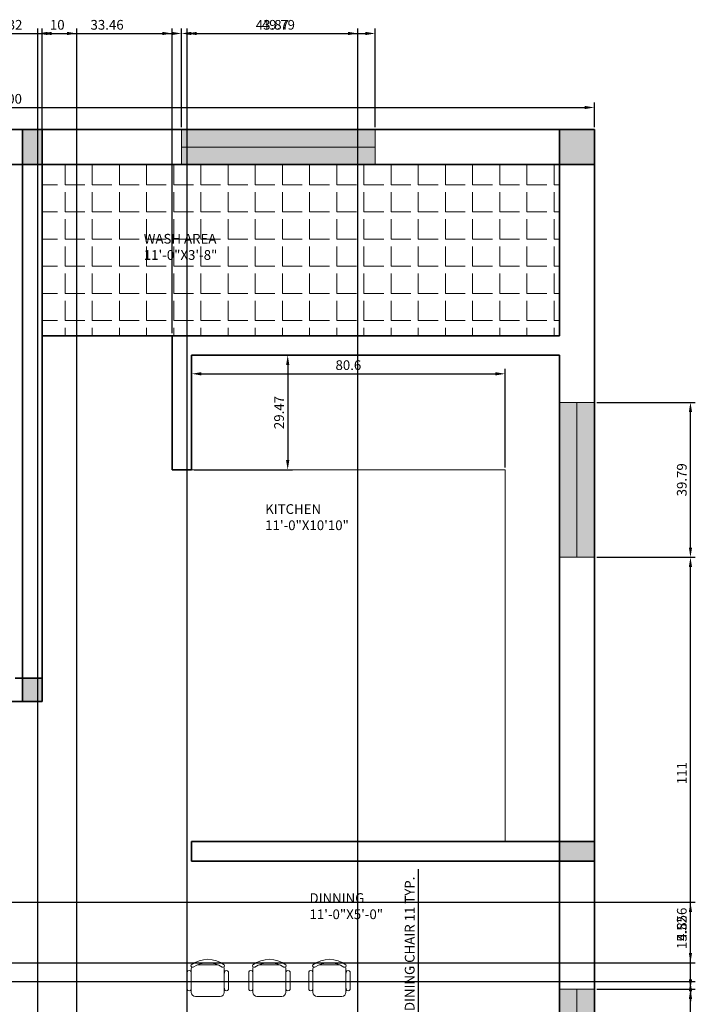
# Model space of a CAD drawing. Units: inches. Extents: x 33934 to 34340, y 20959 to 21493.
# Tile 4 of 4: x 34166 to 34340, y 21240 to 21493. Entities that reach past the tile are written whole.
import ezdxf

# ---------------------------------------------------------------- set-up
doc = ezdxf.new("R2010")
doc.units = ezdxf.units.IN
for name, color, linetype, lineweight in [('A-ANNO-DIMS', 2, 'Continuous', 18), ('A-AREA-IDEN', 7, 'Continuous', 18), ('A-FLOR-CASE', 9, 'Continuous', 18), ('A-FURN', 8, 'Continuous', 18), ('A-GLAZ', 4, 'Continuous', 18), ('A-WALL', 7, 'Continuous', 35)]:
    doc.layers.add(name, color=color, linetype=linetype, lineweight=lineweight)
for name, color, linetype, lineweight, true_color in [('A-COLS-PATT', 141, 'Continuous', 13, 0xadddf7), ('A-FLOR-PATT', 141, 'Continuous', 13, 0xadddf7), ('A-GLAZ-PATT', 159, 'Continuous', 13, 0x22346e)]:
    doc.layers.add(name, color=color, linetype=linetype, lineweight=lineweight, true_color=true_color)
doc.styles.get("Standard").update_dxf_attribs({"font": 'arial.ttf'})
doc.dimstyles.new('ISO-25', dxfattribs={"dimtxt": 2.5, "dimasz": 2.5, "dimexe": 1.25, "dimexo": 0.625, "dimtad": 1, "dimtxsty": 'Standard', "dimcen": 2.5, "dimadec": 0, "dimazin": 0, "dimtfac": 1, "dimtmove": 0, "dimatfit": 3, "dimfxl": 1, "dimarcsym": 0})

# ---------------------------------------------------------------- blocks, each defined once
blk = doc.blocks.new('CHAIR7')
for p, q in [((5.12, 15.04), (17.88, 15.04)), ((0, 9), (0, -9)), ((20, 12), (3, 12)), ((23, -7.44), (23, 7.44)), ((3, -12), (20, -12)), ((5.12, -15), (17.88, -15))]:
    blk.add_line(p, q)
for centre, radius, start, end in [((5.56, 13.54), 1.56, 73.7398, 286.2602), ((17.44, 13.54), 1.56, 253.7398, 106.2602), ((3, 9), 3, 90, 180), ((20, 9), 3, 62.41556, 90), ((22.34, 11.12), 1.1, 53.30994, 212.02741), ((4.82, 0), 19.64, 327.57575, 32.42425), ((7, 0), 20, 323.1301, 36.8699), ((3, -9), 3, 180, 270), ((5.56, -13.5), 1.56, 73.7398, 286.2602), ((17.44, -13.5), 1.56, 253.7398, 106.2602), ((20, -9), 3, 270, 297.58444), ((22.34, -11.12), 1.1, 147.97259, 306.69006)]:
    blk.add_arc(centre, radius, start, end)
blk = doc.blocks.new('*D6')
at = {"layer": 'A-ANNO-DIMS', "color": 0, "lineweight": -2, "transparency": 16777216}
for p, q in [((34013.69, 21465.74), (34013.69, 21472.03)), ((34313.69, 21465.74), (34313.69, 21472.03)), ((34016.19, 21470.78), (34311.19, 21470.78))]:
    blk.add_line(p, q, dxfattribs=at)
at = {"layer": 'A-ANNO-DIMS', "color": 0, "transparency": 16777216}
for points in [[(34016.19, 21471.2), (34016.19, 21470.37), (34013.69, 21470.78)], [(34311.19, 21471.2), (34311.19, 21470.37), (34313.69, 21470.78)]]:
    blk.add_solid(points, dxfattribs=at)
at = {"layer": 'Defpoints', "color": 0, "transparency": 16777216}
for p in [(34313.69, 21470.78), (34013.69, 21465.11), (34313.69, 21465.11)]:
    blk.add_point(p, dxfattribs=at)
at = {"layer": 'A-ANNO-DIMS', "color": 0, "transparency": 16777216, "insert": (34163.69, 21472.69), "char_height": 2.5, "attachment_point": 5}
blk.add_mtext('300', dxfattribs=at)
blk = doc.blocks.new('*D11')
at = {"layer": 'A-ANNO-DIMS', "color": 0, "lineweight": -2, "transparency": 16777216}
for p, q in [((34268.45, 21234.15), (34268.45, 21274.98)), ((34267.46, 21234.15), (34269.7, 21234.15)), ((34268.45, 21225.89), (34268.45, 21231.65)), ((34267.46, 21223.39), (34269.7, 21223.39))]:
    blk.add_line(p, q, dxfattribs=at)
at = {"layer": 'A-ANNO-DIMS', "color": 0, "transparency": 16777216}
for points in [[(34268.03, 21231.65), (34268.87, 21231.65), (34268.45, 21234.15)], [(34268.03, 21225.89), (34268.87, 21225.89), (34268.45, 21223.39)]]:
    blk.add_solid(points, dxfattribs=at)
at = {"layer": 'Defpoints', "color": 0, "transparency": 16777216}
for p in [(34266.83, 21234.15), (34268.45, 21234.15), (34266.83, 21223.39)]:
    blk.add_point(p, dxfattribs=at)
at = {"layer": 'A-ANNO-DIMS', "color": 0, "transparency": 16777216, "insert": (34266.53, 21255.82), "char_height": 2.5, "attachment_point": 5, "rotation": 90}
blk.add_mtext('DINING CHAIR 11 TYP.', dxfattribs=at)
blk = doc.blocks.new('*D15')
at = {"layer": 'A-ANNO-DIMS', "color": 0, "lineweight": -2, "transparency": 16777216}
for p, q in [((34117.23, 21465.74), (34117.23, 21491.06)), ((34119.73, 21489.81), (34205.05, 21489.81)), ((34207.55, 21465.74), (34207.55, 21491.06))]:
    blk.add_line(p, q, dxfattribs=at)
at = {"layer": 'A-ANNO-DIMS', "color": 0, "transparency": 16777216}
for points in [[(34119.73, 21490.23), (34119.73, 21489.39), (34117.23, 21489.81)], [(34205.05, 21490.23), (34205.05, 21489.39), (34207.55, 21489.81)]]:
    blk.add_solid(points, dxfattribs=at)
at = {"layer": 'Defpoints', "color": 0, "transparency": 16777216}
for p in [(34207.55, 21489.81), (34117.23, 21465.11), (34207.55, 21465.11)]:
    blk.add_point(p, dxfattribs=at)
at = {"layer": 'A-ANNO-DIMS', "color": 0, "transparency": 16777216, "insert": (34162.39, 21491.71), "char_height": 2.5, "attachment_point": 5}
blk.add_mtext('90.32', dxfattribs=at)
blk = doc.blocks.new('*D16')
at = {"layer": 'A-ANNO-DIMS', "color": 0, "lineweight": -2, "transparency": 16777216}
for p, q in [((34207.55, 21465.74), (34207.55, 21491.06)), ((34210.05, 21489.81), (34254.84, 21489.81)), ((34257.34, 21465.74), (34257.34, 21491.06))]:
    blk.add_line(p, q, dxfattribs=at)
at = {"layer": 'A-ANNO-DIMS', "color": 0, "transparency": 16777216}
for points in [[(34210.05, 21490.23), (34210.05, 21489.39), (34207.55, 21489.81)], [(34254.84, 21490.23), (34254.84, 21489.39), (34257.34, 21489.81)]]:
    blk.add_solid(points, dxfattribs=at)
at = {"layer": 'Defpoints', "color": 0, "transparency": 16777216}
for p in [(34257.34, 21489.81), (34207.55, 21465.11), (34257.34, 21465.11)]:
    blk.add_point(p, dxfattribs=at)
at = {"layer": 'A-ANNO-DIMS', "color": 0, "transparency": 16777216, "insert": (34232.45, 21491.71), "char_height": 2.5, "attachment_point": 5}
blk.add_mtext('49.79', dxfattribs=at)
blk = doc.blocks.new('*D26')
at = {"layer": 'A-ANNO-DIMS', "color": 0, "lineweight": -2, "transparency": 16777216}
for p, q in [((34314.32, 21244.18), (34339.64, 21244.18)), ((34338.39, 21215.19), (34338.39, 21241.68)), ((34314.32, 21212.69), (34339.64, 21212.69))]:
    blk.add_line(p, q, dxfattribs=at)
at = {"layer": 'A-ANNO-DIMS', "color": 0, "transparency": 16777216}
for points in [[(34337.98, 21241.68), (34338.81, 21241.68), (34338.39, 21244.18)], [(34337.98, 21215.19), (34338.81, 21215.19), (34338.39, 21212.69)]]:
    blk.add_solid(points, dxfattribs=at)
at = {"layer": 'Defpoints', "color": 0, "transparency": 16777216}
for p in [(34313.69, 21244.18), (34338.39, 21244.18), (34313.69, 21212.69)]:
    blk.add_point(p, dxfattribs=at)
at = {"layer": 'A-ANNO-DIMS', "color": 0, "transparency": 16777216, "insert": (34336.49, 21228.44), "char_height": 2.5, "attachment_point": 5, "rotation": 90}
blk.add_mtext('31.496', dxfattribs=at)
blk = doc.blocks.new('*D27')
at = {"layer": 'A-ANNO-DIMS', "color": 0, "lineweight": -2, "transparency": 16777216}
for p, q in [((34314.32, 21355.19), (34339.64, 21355.19)), ((34338.39, 21246.68), (34338.39, 21352.69)), ((34314.32, 21244.18), (34339.64, 21244.18))]:
    blk.add_line(p, q, dxfattribs=at)
at = {"layer": 'A-ANNO-DIMS', "color": 0, "transparency": 16777216}
for points in [[(34337.98, 21352.69), (34338.81, 21352.69), (34338.39, 21355.19)], [(34337.98, 21246.68), (34338.81, 21246.68), (34338.39, 21244.18)]]:
    blk.add_solid(points, dxfattribs=at)
at = {"layer": 'Defpoints', "color": 0, "transparency": 16777216}
for p in [(34313.69, 21355.19), (34338.39, 21355.19), (34313.69, 21244.18)]:
    blk.add_point(p, dxfattribs=at)
at = {"layer": 'A-ANNO-DIMS', "color": 0, "transparency": 16777216, "insert": (34336.51, 21299.69), "char_height": 2.5, "attachment_point": 5, "rotation": 90}
blk.add_mtext('111', dxfattribs=at)
blk = doc.blocks.new('*D28')
at = {"layer": 'A-ANNO-DIMS', "color": 0, "lineweight": -2, "transparency": 16777216}
for p, q in [((34314.32, 21394.98), (34339.64, 21394.98)), ((34338.39, 21357.69), (34338.39, 21392.48)), ((34314.32, 21355.19), (34339.64, 21355.19))]:
    blk.add_line(p, q, dxfattribs=at)
at = {"layer": 'A-ANNO-DIMS', "color": 0, "transparency": 16777216}
for points in [[(34337.98, 21392.48), (34338.81, 21392.48), (34338.39, 21394.98)], [(34337.98, 21357.69), (34338.81, 21357.69), (34338.39, 21355.19)]]:
    blk.add_solid(points, dxfattribs=at)
at = {"layer": 'Defpoints', "color": 0, "transparency": 16777216}
for p in [(34313.69, 21394.98), (34338.39, 21394.98), (34313.69, 21355.19)]:
    blk.add_point(p, dxfattribs=at)
at = {"layer": 'A-ANNO-DIMS', "color": 0, "transparency": 16777216, "insert": (34336.49, 21375.09), "char_height": 2.5, "attachment_point": 5, "rotation": 90}
blk.add_mtext('39.79', dxfattribs=at)
blk = doc.blocks.new('*D33')
at = {"layer": 'A-ANNO-DIMS', "color": 0, "lineweight": -2, "transparency": 16777216}
for p, q in [((34170.61, 21072.74), (34170.61, 21491.06)), ((34173.11, 21489.81), (34178.11, 21489.81)), ((34180.61, 21072.74), (34180.61, 21491.06))]:
    blk.add_line(p, q, dxfattribs=at)
at = {"layer": 'A-ANNO-DIMS', "color": 0, "transparency": 16777216}
for points in [[(34173.11, 21490.23), (34173.11, 21489.39), (34170.61, 21489.81)], [(34178.11, 21490.23), (34178.11, 21489.39), (34180.61, 21489.81)]]:
    blk.add_solid(points, dxfattribs=at)
at = {"layer": 'Defpoints', "color": 0, "transparency": 16777216}
for p in [(34180.61, 21489.81), (34170.61, 21072.11), (34180.61, 21072.11)]:
    blk.add_point(p, dxfattribs=at)
at = {"layer": 'A-ANNO-DIMS', "color": 0, "transparency": 16777216, "insert": (34175.61, 21491.71), "char_height": 2.5, "attachment_point": 5}
blk.add_mtext('10', dxfattribs=at)
blk = doc.blocks.new('*D36')
at = {"layer": 'A-ANNO-DIMS', "color": 0, "lineweight": -2, "transparency": 16777216}
for p, q in [((34208.98, 21220.05), (34208.98, 21491.06)), ((34211.48, 21489.81), (34250.35, 21489.81)), ((34252.85, 21220.05), (34252.85, 21491.06))]:
    blk.add_line(p, q, dxfattribs=at)
at = {"layer": 'A-ANNO-DIMS', "color": 0, "transparency": 16777216}
for points in [[(34211.48, 21490.23), (34211.48, 21489.39), (34208.98, 21489.81)], [(34250.35, 21490.23), (34250.35, 21489.39), (34252.85, 21489.81)]]:
    blk.add_solid(points, dxfattribs=at)
at = {"layer": 'Defpoints', "color": 0, "transparency": 16777216}
for p in [(34252.85, 21489.81), (34208.98, 21219.43), (34252.85, 21219.43)]:
    blk.add_point(p, dxfattribs=at)
at = {"layer": 'A-ANNO-DIMS', "color": 0, "transparency": 16777216, "insert": (34230.91, 21491.71), "char_height": 2.5, "attachment_point": 5}
blk.add_mtext('43.87', dxfattribs=at)
blk = doc.blocks.new('*D42')
at = {"layer": 'A-ANNO-DIMS', "color": 0, "lineweight": -2, "transparency": 16777216}
for p, q in [((34171.69, 21412.74), (34171.69, 21491.06)), ((34174.19, 21489.81), (34202.65, 21489.81)), ((34205.15, 21412.74), (34205.15, 21491.06))]:
    blk.add_line(p, q, dxfattribs=at)
at = {"layer": 'A-ANNO-DIMS', "color": 0, "transparency": 16777216}
for points in [[(34174.19, 21490.23), (34174.19, 21489.39), (34171.69, 21489.81)], [(34202.65, 21490.23), (34202.65, 21489.39), (34205.15, 21489.81)]]:
    blk.add_solid(points, dxfattribs=at)
at = {"layer": 'Defpoints', "color": 0, "transparency": 16777216}
for p in [(34205.15, 21489.81), (34171.69, 21412.11), (34205.15, 21412.11)]:
    blk.add_point(p, dxfattribs=at)
at = {"layer": 'A-ANNO-DIMS', "color": 0, "transparency": 16777216, "insert": (34188.42, 21491.71), "char_height": 2.5, "attachment_point": 5}
blk.add_mtext('33.46', dxfattribs=at)
blk = doc.blocks.new('*D46')
at = {"layer": 'A-ANNO-DIMS', "color": 0, "lineweight": -2, "transparency": 16777216}
for p, q in [((34116.25, 21266.49), (34339.64, 21266.49)), ((34338.39, 21253.47), (34338.39, 21263.99)), ((34116.25, 21250.97), (34339.64, 21250.97))]:
    blk.add_line(p, q, dxfattribs=at)
at = {"layer": 'A-ANNO-DIMS', "color": 0, "transparency": 16777216}
for points in [[(34337.98, 21263.99), (34338.81, 21263.99), (34338.39, 21266.49)], [(34337.98, 21253.47), (34338.81, 21253.47), (34338.39, 21250.97)]]:
    blk.add_solid(points, dxfattribs=at)
at = {"layer": 'Defpoints', "color": 0, "transparency": 16777216}
for p in [(34115.62, 21266.49), (34338.39, 21266.49), (34115.62, 21250.97)]:
    blk.add_point(p, dxfattribs=at)
at = {"layer": 'A-ANNO-DIMS', "color": 0, "transparency": 16777216, "insert": (34336.49, 21258.73), "char_height": 2.5, "attachment_point": 5, "rotation": 90}
blk.add_mtext('15.52', dxfattribs=at)
blk = doc.blocks.new('*D47')
at = {"layer": 'A-ANNO-DIMS', "color": 0, "lineweight": -2, "transparency": 16777216}
for p, q in [((34338.39, 21253.47), (34338.39, 21265.75)), ((34116.25, 21250.97), (34339.64, 21250.97)), ((34338.39, 21246.11), (34338.39, 21250.97)), ((34116.32, 21246.11), (34339.64, 21246.11)), ((34338.39, 21243.61), (34338.39, 21241.11))]:
    blk.add_line(p, q, dxfattribs=at)
at = {"layer": 'A-ANNO-DIMS', "color": 0, "transparency": 16777216}
for points in [[(34337.98, 21253.47), (34338.81, 21253.47), (34338.39, 21250.97)], [(34337.98, 21243.61), (34338.81, 21243.61), (34338.39, 21246.11)]]:
    blk.add_solid(points, dxfattribs=at)
at = {"layer": 'Defpoints', "color": 0, "transparency": 16777216}
for p in [(34115.62, 21250.97), (34338.39, 21250.97), (34115.69, 21246.11)]:
    blk.add_point(p, dxfattribs=at)
at = {"layer": 'A-ANNO-DIMS', "color": 0, "transparency": 16777216, "insert": (34336.49, 21260.86), "char_height": 2.5, "attachment_point": 5, "rotation": 90}
blk.add_mtext('4.856', dxfattribs=at)
blk = doc.blocks.new('*D52')
at = {"layer": 'A-ANNO-DIMS', "color": 0, "lineweight": -2, "transparency": 16777216}
for p, q in [((34210.78, 21407.11), (34236.1, 21407.11)), ((34234.85, 21404.61), (34234.85, 21380.14)), ((34210.78, 21377.64), (34236.1, 21377.64))]:
    blk.add_line(p, q, dxfattribs=at)
at = {"layer": 'A-ANNO-DIMS', "color": 0, "transparency": 16777216}
for points in [[(34234.44, 21404.61), (34235.27, 21404.61), (34234.85, 21407.11)], [(34234.44, 21380.14), (34235.27, 21380.14), (34234.85, 21377.64)]]:
    blk.add_solid(points, dxfattribs=at)
at = {"layer": 'Defpoints', "color": 0, "transparency": 16777216}
for p in [(34210.15, 21407.11), (34210.15, 21377.64), (34234.85, 21377.64)]:
    blk.add_point(p, dxfattribs=at)
at = {"layer": 'A-ANNO-DIMS', "color": 0, "transparency": 16777216, "insert": (34232.95, 21392.38), "char_height": 2.5, "attachment_point": 5, "rotation": 90}
blk.add_mtext('29.47', dxfattribs=at)
blk = doc.blocks.new('*D53')
at = {"layer": 'A-ANNO-DIMS', "color": 0, "lineweight": -2, "transparency": 16777216}
for p, q in [((34210.15, 21378.27), (34210.15, 21403.59)), ((34290.75, 21378.27), (34290.75, 21403.59)), ((34212.65, 21402.34), (34288.25, 21402.34))]:
    blk.add_line(p, q, dxfattribs=at)
at = {"layer": 'A-ANNO-DIMS', "color": 0, "transparency": 16777216}
for points in [[(34212.65, 21402.76), (34212.65, 21401.92), (34210.15, 21402.34)], [(34288.25, 21402.76), (34288.25, 21401.92), (34290.75, 21402.34)]]:
    blk.add_solid(points, dxfattribs=at)
at = {"layer": 'Defpoints', "color": 0, "transparency": 16777216}
for p in [(34290.75, 21402.34), (34210.15, 21377.64), (34290.75, 21377.64)]:
    blk.add_point(p, dxfattribs=at)
at = {"layer": 'A-ANNO-DIMS', "color": 0, "transparency": 16777216, "insert": (34250.45, 21404.24), "char_height": 2.5, "attachment_point": 5}
blk.add_mtext('80.6', dxfattribs=at)

msp = doc.modelspace()

# ---------------------------------------------------------------- hatches: boundary and pattern name
at = {"layer": 'A-COLS-PATT'}
h = msp.add_hatch(color=256, dxfattribs=at)
h.dxf.hatch_style = 1
h.paths.add_polyline_path([(34022.6921, 20994.1104), (34013.6921, 20994.1104), (34013.6921, 20985.1104), (34022.6921, 20985.1104)])
h.paths.add_polyline_path([(34163.6921, 20994.1104), (34158.6922, 20994.1104), (34158.6922, 20985.1104), (34163.6921, 20985.1104)])
h.paths.add_polyline_path([(34313.6921, 20994.1104), (34304.6921, 20994.1104), (34304.6921, 20985.1104), (34313.6921, 20985.1104)])
h.paths.add_polyline_path([(34313.6921, 21077.1104), (34304.6921, 21077.1104), (34304.6921, 21072.1104), (34313.6921, 21072.1104)])
h.paths.add_polyline_path([(34172.6921, 21077.1104), (34167.6921, 21077.1104), (34167.6921, 21072.1104), (34172.6921, 21072.1104)])
h.paths.add_polyline_path([(34022.6921, 21324.1104), (34013.6921, 21324.1104), (34013.6921, 21318.1104), (34022.6921, 21318.1104)])
h.paths.add_polyline_path([(34171.6921, 21324.1104), (34166.6921, 21324.1104), (34166.6921, 21318.1104), (34171.6921, 21318.1104)])
h.paths.add_polyline_path([(34313.6921, 21282.1104), (34304.6921, 21282.1104), (34304.6921, 21277.1104), (34313.6921, 21277.1104)])
h.paths.add_polyline_path([(34313.6921, 21465.1104), (34304.6921, 21465.1104), (34304.6921, 21456.1104), (34313.6921, 21456.1104)])
h.paths.add_polyline_path([(34171.6921, 21465.1104), (34166.6921, 21465.1104), (34166.6921, 21456.1104), (34171.6921, 21456.1104)])
h.paths.add_polyline_path([(34022.6921, 21465.1104), (34013.6921, 21465.1104), (34013.6921, 21456.1104), (34022.6921, 21456.1104)])
at = {"layer": 'A-FLOR-PATT'}
h = msp.add_hatch(dxfattribs=at)
h.set_pattern_fill('ANGLE', color=256)
h.set_pattern_definition([(0, (0, 0), (0, 6.985), [5.08, -1.905]), (90, (0, 0), (-6.985, 4e-16), [5.08, -1.905])])
h.paths.add_polyline_path([(34304.6921, 21456.1104), (34171.6921, 21456.1104), (34171.6921, 21412.1104), (34202.5687, 21412.1104), (34304.6921, 21412.1104)])
at = {"layer": 'A-GLAZ-PATT'}
h = msp.add_hatch(color=256, dxfattribs=at)
h.dxf.hatch_style = 1
h.paths.add_polyline_path([(34022.6921, 21212.6089), (34018.1921, 21212.6089), (34018.1921, 21149.8921), (34022.6921, 21149.8921)])
h.paths.add_polyline_path([(34018.1921, 21212.6089), (34013.6921, 21212.6089), (34013.6921, 21149.8921), (34018.1921, 21149.8921)])
h.paths.add_polyline_path([(34142.0454, 21077.1104), (34099.5314, 21077.1104), (34099.5314, 21074.6104), (34142.0454, 21074.6104)])
h.paths.add_polyline_path([(34142.0454, 21074.6104), (34099.5314, 21074.6104), (34099.5314, 21072.1104), (34142.0454, 21072.1104)])
h.paths.add_polyline_path([(34313.6921, 21160.1148), (34309.1921, 21160.1148), (34309.1921, 21107.9155), (34313.6921, 21107.9155)])
h.paths.add_polyline_path([(34309.1921, 21160.1148), (34304.6921, 21160.1148), (34304.6921, 21107.9155), (34309.1921, 21107.9155)])
h.paths.add_polyline_path([(34309.1921, 21244.1846), (34304.6921, 21244.1846), (34304.6921, 21212.6883), (34309.1921, 21212.6883)])
h.paths.add_polyline_path([(34313.6921, 21244.1846), (34309.1921, 21244.1846), (34309.1921, 21212.6883), (34313.6921, 21212.6883)])
h.paths.add_polyline_path([(34313.6921, 21394.9809), (34309.1921, 21394.9809), (34309.1921, 21355.1902), (34313.6921, 21355.1902)])
h.paths.add_polyline_path([(34309.1921, 21394.9809), (34304.6921, 21394.9809), (34304.6921, 21355.1902), (34309.1921, 21355.1902)])
h.paths.add_polyline_path([(34257.3396, 21465.1104), (34207.5515, 21465.1104), (34207.5515, 21460.6104), (34257.3396, 21460.6104)])
h.paths.add_polyline_path([(34257.3396, 21460.6104), (34207.5515, 21460.6104), (34207.5515, 21456.1104), (34257.3396, 21456.1104)])
h.paths.add_polyline_path([(34117.2268, 21465.1104), (34063.6855, 21465.1104), (34063.6855, 21460.6104), (34117.2268, 21460.6104)])
h.paths.add_polyline_path([(34117.2268, 21460.6104), (34063.6855, 21460.6104), (34063.6855, 21456.1104), (34117.2268, 21456.1104)])
h.paths.add_polyline_path([(34022.6921, 21430.8215), (34018.1921, 21430.8215), (34018.1921, 21373.469), (34022.6921, 21373.469)])
h.paths.add_polyline_path([(34018.1921, 21430.8215), (34013.6921, 21430.8215), (34013.6921, 21373.469), (34018.1921, 21373.469)])
h.paths.add_polyline_path([(34018.1921, 21305.2021), (34013.6921, 21305.2021), (34013.6921, 21272.8905), (34018.1921, 21272.8905)])
h.paths.add_polyline_path([(34022.6921, 21305.2021), (34018.1921, 21305.2021), (34018.1921, 21272.8905), (34022.6921, 21272.8905)])

# ---------------------------------------------------------------- linework, layer by layer
at = {"layer": 'A-FLOR-CASE'}
for p, q in [((34210.1528, 21377.6405), (34290.7503, 21377.6405)), ((34290.7503, 21377.6405), (34290.7503, 21336.1104)), ((34290.7503, 21336.1104), (34290.7503, 21282.1104))]:
    msp.add_line(p, q, dxfattribs=at)
at = {"layer": 'A-GLAZ'}
for p, q in [((34207.5515, 21465.1104), (34207.5515, 21456.1104)), ((34257.3396, 21465.1104), (34207.5515, 21465.1104)), ((34207.5515, 21465.1104), (34207.5515, 21460.6104)), ((34257.3396, 21456.1104), (34257.3396, 21465.1104)), ((34207.5515, 21460.6104), (34257.3396, 21460.6104)), ((34207.5515, 21456.1104), (34257.3396, 21456.1104)), ((34304.6921, 21394.9809), (34313.6921, 21394.9809)), ((34309.1921, 21355.1902), (34309.1921, 21394.9809)), ((34313.6921, 21394.9809), (34313.6921, 21355.1902)), ((34313.6921, 21355.1902), (34304.6921, 21355.1902)), ((34304.6921, 21355.1902), (34309.1921, 21355.1902)), ((34304.6921, 21244.1846), (34313.6921, 21244.1846)), ((34309.1921, 21212.6883), (34309.1921, 21244.1846)), ((34313.6921, 21244.1846), (34313.6921, 21212.6883))]:
    msp.add_line(p, q, dxfattribs=at)
at = {"layer": 'A-WALL'}
for p, q in [((34013.6921, 21465.1104), (34313.6921, 21465.1104)), ((34166.6921, 21318.1104), (34166.6921, 21465.1104)), ((34171.6921, 21412.1104), (34171.6921, 21465.1104)), ((34304.6921, 21465.1104), (34304.6921, 21412.1104)), ((34313.6921, 21465.1104), (34313.6921, 20985.1104)), ((34013.6921, 21456.1104), (34313.6921, 21456.1104)), ((34171.6921, 21412.1104), (34202.5687, 21412.1104)), ((34171.6921, 21336.1104), (34171.6921, 21412.1104)), ((34304.6921, 21412.1104), (34202.5687, 21412.1104)), ((34205.1528, 21377.6405), (34205.1528, 21412.1104)), ((34277.7183, 21412.1104), (34304.6921, 21412.1104)), ((34277.7183, 21407.1104), (34210.1528, 21407.1104)), ((34210.1528, 21407.1104), (34210.1528, 21377.6405)), ((34277.7183, 21407.1104), (34304.6921, 21407.1104)), ((34304.6921, 21407.1104), (34304.6921, 21336.1104)), ((34210.1528, 21377.6405), (34205.1528, 21377.6405)), ((34171.6921, 21318.1104), (34171.6921, 21336.1104)), ((34304.6921, 21336.1104), (34304.6921, 21244.1846)), ((34164.7827, 21324.1104), (34171.6921, 21324.1104)), ((34115.6921, 21318.1104), (34166.6921, 21318.1104)), ((34166.6921, 21318.1104), (34171.6921, 21318.1104)), ((34210.1528, 21277.1104), (34210.1528, 21282.1104)), ((34210.1528, 21282.1104), (34313.6921, 21282.1104)), ((34277.7183, 21277.1104), (34210.1528, 21277.1104)), ((34277.7183, 21277.1104), (34313.6921, 21277.1104)), ((34304.6921, 21257.1104), (34304.6921, 20985.1104))]:
    msp.add_line(p, q, dxfattribs=at)

# ---------------------------------------------------------------- block references
at = {"layer": 'A-FURN', "xscale": -0.353847974837975, "yscale": 0.353847974837975, "zscale": 0.353847974837975, "rotation": 270}
for p in [(34214.3027, 21242.2855), (34230.1325, 21242.2855), (34245.5813, 21242.2855)]:
    msp.add_blockref('CHAIR7', p, dxfattribs=at)

# ---------------------------------------------------------------- texts
at = {"layer": 'A-AREA-IDEN', "char_height": 2.5, "attachment_point": 1}
for s, width, insert in [('WASH AREA\\P11\'-0"X3\'-8"', 26.592523, (34197.8523, 21438.297)), ('KITCHEN\\P11\'-0"X10\'10"', 54.927079, (34229.0595, 21368.822)), ('DINNING\\P11\'-0"X5\'-0"', 45.517094, (34240.4545, 21268.8336))]:
    msp.add_mtext_dynamic_manual_height_columns(s, width=width, gutter_width=12.5, heights=[0], dxfattribs=dict(at, insert=insert))

# ---------------------------------------------------------------- dimensions: what is measured, and where the dimension line sits
at = {"layer": 'A-ANNO-DIMS'}
for base, p1, p2, override, picture, middle in [((34207.5515, 21489.8104), (34117.2268, 21465.1104), (34207.5515, 21465.1104), {"dimdec": 2, "dimlfac": 1, "dimrnd": 0, "dimzin": 0, "dimdsep": 46, "dimlunit": 2}, '*D15', (34162.3892, 21491.7127)), ((34180.6062, 21489.8104), (34170.6062, 21072.1104), (34180.6062, 21072.1104), {"dimdec": 0, "dimlfac": 1, "dimrnd": 0, "dimzin": 0, "dimdsep": 46, "dimlunit": 2}, '*D33', (34175.6062, 21491.7119)), ((34205.1528, 21489.8104), (34171.6921, 21412.1104), (34205.1528, 21412.1104), {"dimdec": 2, "dimlfac": 1, "dimrnd": 0, "dimzin": 0, "dimdsep": 46, "dimlunit": 2}, '*D42', (34188.4225, 21491.7127)), ((34257.3396, 21489.8104), (34207.5515, 21465.1104), (34257.3396, 21465.1104), {"dimdec": 2, "dimlfac": 1, "dimrnd": 0, "dimzin": 0, "dimdsep": 46, "dimlunit": 2}, '*D16', (34232.4456, 21491.7119)), ((34252.8454, 21489.8104), (34208.9796, 21219.4265), (34252.8454, 21219.4265), {"dimdec": 2, "dimlfac": 1, "dimrnd": 0, "dimzin": 0, "dimdsep": 46, "dimlunit": 2}, '*D36', (34230.9125, 21491.7127)), ((34313.6921, 21470.7844), (34013.6921, 21465.1104), (34313.6921, 21465.1104), {"dimclrd": 0, "dimclre": 0, "dimclrt": 0}, '*D6', (34163.6921, 21472.6867)), ((34290.7503, 21402.3405), (34210.1528, 21377.6405), (34290.7503, 21377.6405), {"dimdec": 1, "dimlfac": 1, "dimrnd": 0, "dimzin": 0, "dimdsep": 46, "dimlunit": 2}, '*D53', (34250.4516, 21404.242))]:
    dim = msp.add_linear_dim(base=base, p1=p1, p2=p2, dimstyle='ISO-25', override=override, dxfattribs=at)
    dim.commit()
    dim.dimension.update_dxf_attribs({"geometry": picture, "text_midpoint": middle})
for base, p1, p2, angle, override, picture, middle in [((34234.8528, 21377.6405), (34210.1528, 21407.1104), (34210.1528, 21377.6405), 270, {"dimdec": 2, "dimlfac": 1, "dimrnd": 0, "dimzin": 0, "dimdsep": 46, "dimlunit": 2}, '*D52', (34232.9514, 21392.3755)), ((34338.3921, 21394.9809), (34313.6921, 21355.1902), (34313.6921, 21394.9809), 90, {"dimdec": 2, "dimlfac": 1, "dimrnd": 0, "dimzin": 0, "dimdsep": 46, "dimlunit": 2}, '*D28', (34336.4899, 21375.0856)), ((34338.3921, 21355.1902), (34313.6921, 21244.1846), (34313.6921, 21355.1902), 90, {"dimdec": 0, "dimlfac": 1, "dimrnd": 0, "dimzin": 0, "dimdsep": 46, "dimlunit": 2}, '*D27', (34336.512, 21299.6874)), ((34338.3921, 21266.4872), (34115.6238, 21250.9668), (34115.6238, 21266.4872), 90, {"dimdec": 2, "dimlfac": 1, "dimrnd": 0, "dimzin": 0, "dimdsep": 46, "dimlunit": 2}, '*D46', (34336.4907, 21258.727)), ((34338.3921, 21250.9668), (34115.6921, 21246.1104), (34115.6238, 21250.9668), 90, {"dimdec": 3, "dimlfac": 1, "dimrnd": 0, "dimzin": 0, "dimdsep": 46, "dimlunit": 2}, '*D47', (34336.4907, 21260.8593)), ((34338.3921, 21244.1846), (34313.6921, 21212.6883), (34313.6921, 21244.1846), 90, {"dimdec": 3, "dimlfac": 1, "dimrnd": 0, "dimzin": 0, "dimdsep": 46, "dimlunit": 2}, '*D26', (34336.4899, 21228.4364))]:
    dim = msp.add_linear_dim(base=base, p1=p1, p2=p2, angle=angle, dimstyle='ISO-25', override=override, dxfattribs=at)
    dim.commit()
    dim.dimension.update_dxf_attribs({"geometry": picture, "text_midpoint": middle})
dim = msp.add_linear_dim(base=(34268.4486, 21234.1528), p1=(34266.8342, 21223.3907), p2=(34266.8342, 21234.1528), angle=90, text='DINING CHAIR <> TYP.', dimstyle='ISO-25', override={"dimdec": 0, "dimlfac": 1, "dimrnd": 0, "dimzin": 0, "dimdsep": 46, "dimlunit": 2}, dxfattribs=at)
dim.commit()
dim.dimension.update_dxf_attribs({"geometry": '*D11', "text_midpoint": (34266.5309, 21255.8155)})

doc.saveas('drawing.dxf')
